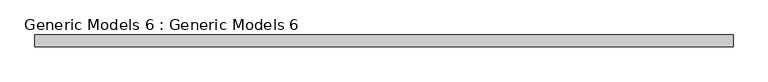
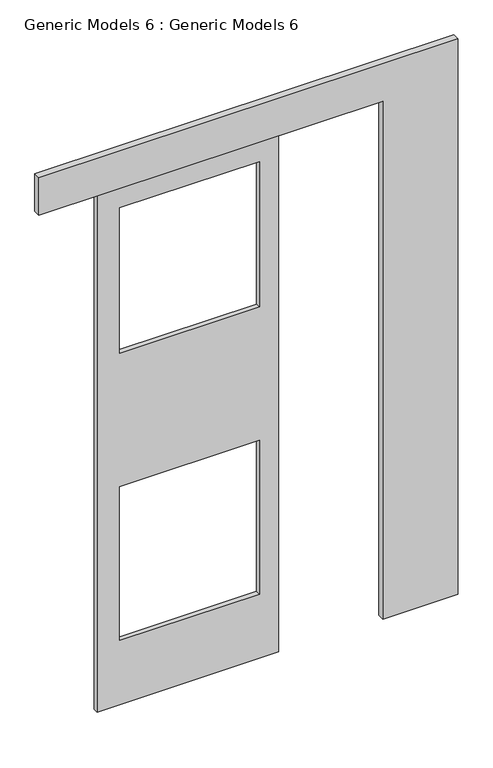
"""IFC4 building model written with IfcOpenShell, lengths in millimetres: proxy geometry, Generic Models 6 : Generic Models 6."""

from ifc_helpers import new_model, si_unit, frame, origin, place, context, project, spatial, polyline, outline, extrude, source, transform, mapped, element, save


def generic_models_6_generic_models_6_7d9998ff(model_context):
    return source(origin(), model_context, "Body", "SweptSolid", [
        extrude(outline(polyline([(5971.6380609, -11539.8503587), (0.0, -11539.8503587), (0.0, -9558.6503587), (5971.6380609, -9558.6503587), (5971.6380609, -11539.8503587)]), holes=[polyline([(5725.9797172, -11292.2003587), (5725.9797172, -9768.2003587), (4050.5645472, -9768.2003587), (4050.5645472, -11292.2003587), (5725.9797172, -11292.2003587)]), polyline([(2511.49538, -9768.2003587), (739.995359, -9768.2003587), (739.995359, -11292.2003587), (2511.49538, -11292.2003587), (2511.49538, -9768.2003587)])]), frame((0.0, -13974.9526331, 0.0), z_axis=(0.0, 1.0, 0.0), x_axis=(0.0, 0.0, 1.0)), (0.0, 0.0, 1.0), 50.8),
        extrude(outline(polyline([(5971.6380609, -8434.7003587), (0.0, -8434.7003587), (0.0, -7615.5503587), (6400.8, -7615.5503587), (6400.8, -12187.5503587), (5971.6380609, -12187.5503587), (5971.6380609, -8434.7003587)])), frame((0.0, -14000.3526331, 0.0), z_axis=(0.0, 1.0, 0.0), x_axis=(0.0, 0.0, 1.0)), (0.0, 0.0, 1.0), 76.2),
    ])


if __name__ == "__main__":
    model = new_model("IFC4")
    model_context = context("Model", 3, world=origin())
    ifc_project = project(units=[si_unit("LENGTHUNIT", "METRE", prefix="MILLI")], contexts=[model_context])
    site = spatial("IfcSite", under=ifc_project)
    building = spatial("IfcBuilding", under=site)
    placement = place(None, origin())
    generic_models_6_generic_models_6_shape = generic_models_6_generic_models_6_7d9998ff(model_context)
    element("IfcBuildingElementProxy", 1, Name="Generic Models 6 : Generic Models 6", ObjectType="Generic Models 6 : Generic Models 6", at=placement, inside=building, context=model_context, shape_type="MappedRepresentation", body=[
        mapped(generic_models_6_generic_models_6_shape, transform((0.0, 0.0, 0.0), x_axis=(1.0, 0.0, 0.0), y_axis=(0.0, 1.0, 0.0), z_axis=(0.0, 0.0, 1.0))),
    ])
    save(model, "model.ifc")
